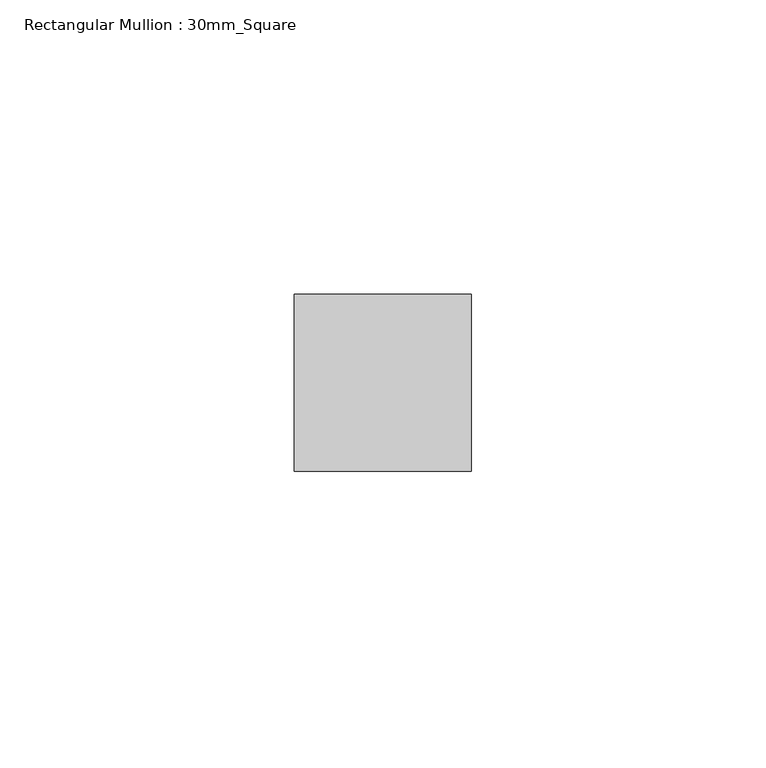
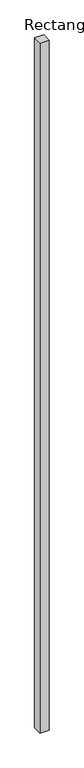
"""IFC4 building model written with IfcOpenShell, lengths in millimetres: member geometry, Rectangular Mullion : 30mm_Square."""

from ifc_helpers import new_model, si_unit, frame, origin, place, context, project, spatial, polyline, outline, extrude, source, transform, mapped, element, save


def rectangular_mullion_30mm_square_9325025b(model_context):
    return source(origin(), model_context, "Body", "SweptSolid", [
        extrude(outline(polyline([(15.0, 15.0), (15.0, -15.0), (-15.0, -15.0), (-15.0, 15.0), (15.0, 15.0)])), frame((0.0, 0.0, -2400.0), z_axis=(0.0, 0.0, 1.0), x_axis=(1.0, 0.0, 0.0)), (0.0, 0.0, 1.0), 2400.0),
    ])


if __name__ == "__main__":
    model = new_model("IFC4")
    model_context = context("Model", 3, world=origin())
    ifc_project = project(units=[si_unit("LENGTHUNIT", "METRE", prefix="MILLI")], contexts=[model_context])
    site = spatial("IfcSite", under=ifc_project)
    building = spatial("IfcBuilding", under=site)
    placement = place(None, origin())
    rectangular_mullion_30mm_square_shape = rectangular_mullion_30mm_square_9325025b(model_context)
    element("IfcMember", 1, ObjectType="Rectangular Mullion : 30mm_Square", at=placement, inside=building, context=model_context, shape_type="MappedRepresentation", body=[
        mapped(rectangular_mullion_30mm_square_shape, transform((0.0, 0.0, 0.0), x_axis=(1.0, 0.0, 0.0), y_axis=(0.0, 1.0, 0.0), z_axis=(0.0, 0.0, 1.0))),
    ])
    save(model, "model.ifc")

# Revit data of these elements
# Type "Rectangular Mullion : 30mm_Square"
#   Keynote = "H11"
#   built-in parameter 1007304 = 0.0984252 (stored number, unit not read)
#   built-in parameter 1007301 = 0.0492126 (stored number, unit not read)
#   built-in parameter 1007300 = 0.0492126 (stored number, unit not read)
# Element 1 (IfcMember, "Rectangular Mullion : 30mm_Square")
#   Materials on its faces: "Aluminium"
# Materials
#   "Aluminium": class "Metal", colour RGB 247 247 247, transparency 0, Description = "Aluminium 6061", Cost = 0
